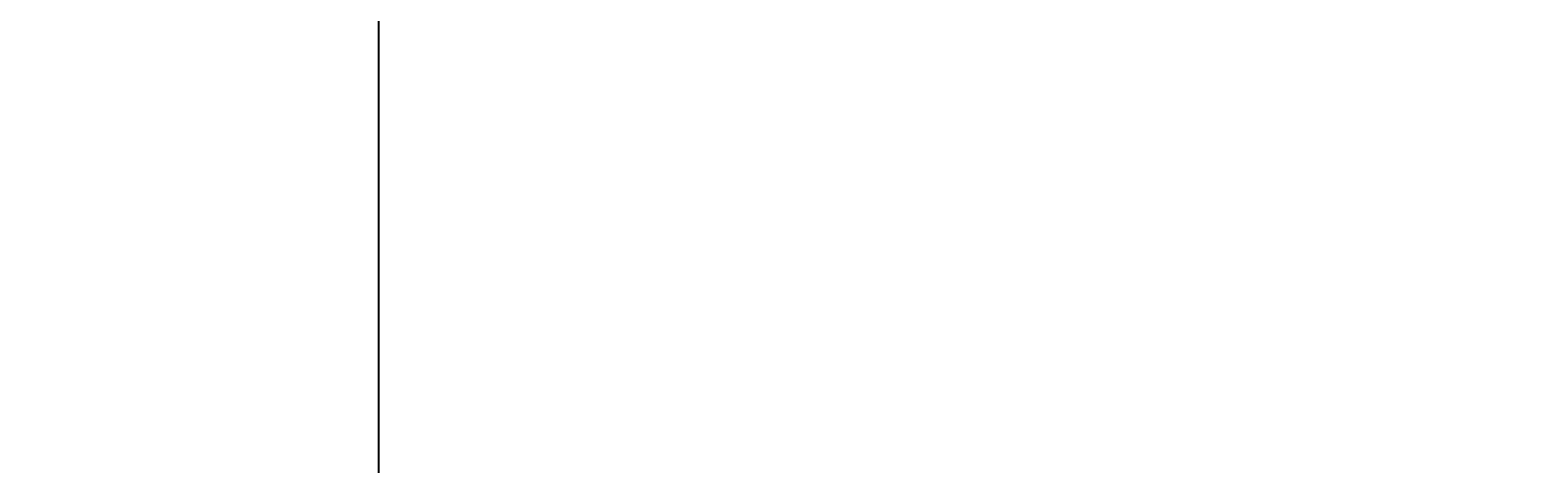
# Model space of a CAD drawing. Units: inches. Extents: x 35362 to 73946, y 43607 to 67532.
# Tile 133 of 134: x 64925 to 66704, y 44948 to 45460. Entities that reach past the tile are written whole.
import ezdxf

# ---------------------------------------------------------------- set-up
doc = ezdxf.new("R2010")
doc.units = ezdxf.units.IN
doc.header["$MEASUREMENT"] = 0
doc.layers.add('A-ANNO-DIMS', color=2, linetype='Continuous', lineweight=18)
doc.styles.get("Standard").update_dxf_attribs({"font": 'arial.ttf'})
doc.dimstyles.get("Standard").update_dxf_attribs({"dimtxt": 0.18, "dimasz": 0.18, "dimexe": 0.18, "dimexo": 0.0625, "dimgap": 0.09, "dimtad": 0, "dimtih": 1, "dimtoh": 1, "dimdec": 4, "dimzin": 0, "dimdsep": 46, "dimtxsty": 'Standard', "dimcen": 0.09, "dimadec": 0, "dimazin": 0, "dimtfac": 1, "dimtdec": 4, "dimtofl": 0, "dimtmove": 0, "dimatfit": 3, "dimfxl": 1, "dimtolj": 1, "dimtzin": 0, "dimarcsym": 0})

# ---------------------------------------------------------------- blocks, each defined once
blk = doc.blocks.new('*D5')
at = {"layer": 'A-ANNO-DIMS', "color": 0, "lineweight": -2, "transparency": 16777216}
for p, q in [((37121.949085, 46919.318283), (37121.949085, 43606.678996)), ((69871.496302, 45449.831951), (69871.496302, 43606.678996)), ((37122.129085, 43606.858996), (53496.2943647142, 43606.858996)), ((69871.316302, 43606.858996), (53497.15102228581, 43606.858996))]:
    blk.add_line(p, q, dxfattribs=at)
at = {"layer": 'A-ANNO-DIMS', "color": 0, "transparency": 16777216}
for points in [[(37122.129085, 43606.888996), (37122.129085, 43606.828996), (37121.949085, 43606.858996)], [(69871.316302, 43606.888996), (69871.316302, 43606.828996), (69871.496302, 43606.858996)]]:
    blk.add_solid(points, dxfattribs=at)
at = {"layer": 'Defpoints', "color": 0, "transparency": 16777216}
for p in [(37121.949085, 46919.380783), (69871.496302, 45449.894451), (69871.496302, 43606.858996)]:
    blk.add_point(p, dxfattribs=at)
at = {"layer": 'A-ANNO-DIMS', "color": 0, "transparency": 16777216, "insert": (53496.7226935, 43606.858996), "char_height": 0.18, "attachment_point": 5}
blk.add_mtext('\\A1;32750', dxfattribs=at)
blk = doc.blocks.new('*D38')
at = {"layer": 'A-ANNO-DIMS', "color": 0, "lineweight": -2, "transparency": 16777216}
for p, q in [((68483.500128, 45449.831951), (68483.500128, 43606.678996)), ((62090.58505699999, 45366.796496), (62090.58505699999, 43606.678996)), ((62090.76505699999, 43606.858996), (65286.57828827081, 43606.858996)), ((68483.320128, 43606.858996), (65287.5068967292, 43606.858996))]:
    blk.add_line(p, q, dxfattribs=at)
at = {"layer": 'A-ANNO-DIMS', "color": 0, "transparency": 16777216}
for points in [[(62090.76505699999, 43606.888996), (62090.76505699999, 43606.828996), (62090.58505699999, 43606.858996)], [(68483.320128, 43606.888996), (68483.320128, 43606.828996), (68483.500128, 43606.858996)]]:
    blk.add_solid(points, dxfattribs=at)
at = {"layer": 'Defpoints', "color": 0, "transparency": 16777216}
for p in [(68483.500128, 45449.894451), (62090.58505699999, 45366.858996), (68483.500128, 43606.858996)]:
    blk.add_point(p, dxfattribs=at)
at = {"layer": 'A-ANNO-DIMS', "color": 0, "transparency": 16777216, "insert": (65287.0425925, 43606.858996), "char_height": 0.18, "attachment_point": 5}
blk.add_mtext('\\A1;6392.9', dxfattribs=at)
blk = doc.blocks.new('*D65')
at = {"layer": 'A-ANNO-DIMS', "color": 0, "lineweight": -2, "transparency": 16777216}
for p, q in [((65336.01600799999, 61293.223552), (65336.01600799999, 43606.678996)), ((67326.639741, 61293.223552), (67326.639741, 43606.678996)), ((65336.19600799999, 43606.858996), (66330.87277900206, 43606.858996)), ((67326.45974100001, 43606.858996), (66331.78296999796, 43606.858996))]:
    blk.add_line(p, q, dxfattribs=at)
at = {"layer": 'A-ANNO-DIMS', "color": 0, "transparency": 16777216}
for points in [[(65336.19600799999, 43606.888996), (65336.19600799999, 43606.828996), (65336.01600799999, 43606.858996)], [(67326.45974100001, 43606.888996), (67326.45974100001, 43606.828996), (67326.639741, 43606.858996)]]:
    blk.add_solid(points, dxfattribs=at)
at = {"layer": 'Defpoints', "color": 0, "transparency": 16777216}
for p in [(65336.01600799999, 61293.286052), (67326.639741, 61293.286052), (67326.639741, 43606.858996)]:
    blk.add_point(p, dxfattribs=at)
at = {"layer": 'A-ANNO-DIMS', "color": 0, "transparency": 16777216, "insert": (66331.32787450001, 43606.858996), "char_height": 0.18, "attachment_point": 5}
blk.add_mtext('\\A1;1990.6', dxfattribs=at)
blk = doc.blocks.new('*D68')
at = {"layer": 'A-ANNO-DIMS', "color": 0, "lineweight": -2, "transparency": 16777216}
for p, q in [((68320.870762, 54372.885224), (68320.870762, 43606.678996)), ((61240.907336, 53351.466162), (61240.907336, 43606.678996)), ((61241.08733599999, 43606.858996), (64780.42646373397, 43606.858996)), ((68320.69076200001, 43606.858996), (64781.35163426603, 43606.858996))]:
    blk.add_line(p, q, dxfattribs=at)
at = {"layer": 'A-ANNO-DIMS', "color": 0, "transparency": 16777216}
for points in [[(61241.08733599999, 43606.888996), (61241.08733599999, 43606.828996), (61240.907336, 43606.858996)], [(68320.69076200001, 43606.888996), (68320.69076200001, 43606.828996), (68320.870762, 43606.858996)]]:
    blk.add_solid(points, dxfattribs=at)
at = {"layer": 'Defpoints', "color": 0, "transparency": 16777216}
for p in [(68320.870762, 54372.947724), (61240.907336, 53351.52866199999), (68320.870762, 43606.858996)]:
    blk.add_point(p, dxfattribs=at)
at = {"layer": 'A-ANNO-DIMS', "color": 0, "transparency": 16777216, "insert": (64780.889049, 43606.858996), "char_height": 0.18, "attachment_point": 5}
blk.add_mtext('\\A1;7080.0', dxfattribs=at)

msp = doc.modelspace()

# ---------------------------------------------------------------- dimensions: what is measured, and where the dimension line sits
at = {"layer": 'A-ANNO-DIMS'}
for base, p1, p2, override, picture, middle in [((67326.639741, 43606.858996), (65336.01600799999, 61293.286052), (67326.639741, 61293.286052), {"dimdec": 1, "dimlfac": 1, "dimrnd": 0, "dimzin": 0, "dimdsep": 46, "dimlunit": 2}, '*D65', (66331.32787450001, 43606.858996)), ((68320.870762, 43606.858996), (61240.907336, 53351.52866199999), (68320.870762, 54372.947724), {"dimdec": 1, "dimlfac": 1, "dimrnd": 0, "dimzin": 0, "dimdsep": 46, "dimlunit": 2}, '*D68', (64780.889049, 43606.858996)), ((69871.496302, 43606.858996), (37121.949085, 46919.380783), (69871.496302, 45449.894451), {"dimdec": 0, "dimlfac": 1, "dimrnd": 0, "dimzin": 0, "dimdsep": 46, "dimlunit": 2}, '*D5', (53496.7226935, 43606.858996)), ((68483.500128, 43606.858996), (62090.58505699999, 45366.858996), (68483.500128, 45449.894451), {"dimdec": 1, "dimlfac": 1, "dimrnd": 0, "dimzin": 0, "dimdsep": 46, "dimlunit": 2}, '*D38', (65287.0425925, 43606.858996))]:
    dim = msp.add_linear_dim(base=base, p1=p1, p2=p2, dimstyle='Standard', override=override, dxfattribs=at)
    dim.commit()
    dim.dimension.update_dxf_attribs({"geometry": picture, "text_midpoint": middle})

doc.saveas('drawing.dxf')
